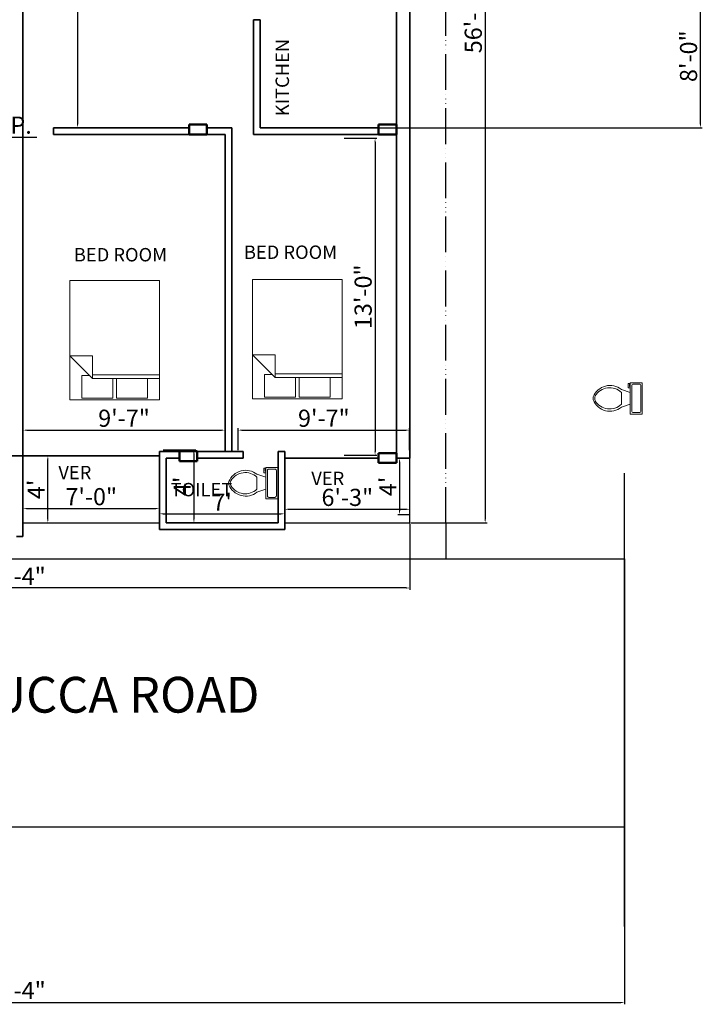
# Model space of a CAD drawing. Units: inches. Extents: x 2680 to 3617, y 1720 to 2823.
# Tile 2 of 4: x 3159 to 3617, y 1720 to 2380. Entities that reach past the tile are written whole.
import ezdxf

# ---------------------------------------------------------------- set-up
doc = ezdxf.new("R2010")
doc.units = ezdxf.units.IN
doc.linetypes.add('ACAD_ISO06W100', pattern=[36, 24, -3, 0, -3, 0, -3, 0, -3])
for name, color, linetype, lineweight in [('A-ANNO-DIMS', 2, 'Continuous', 18), ('A-ANNO-TEXT', 3, 'Continuous', 18), ('A-AREA-IDEN', 244, 'Continuous', 18), ('A-COLS', 1, 'Continuous', 50), ('A-FLOR', 7, 'Continuous', 25), ('A-FLOR-FIXT', 9, 'Continuous', 18), ('A-FURN', 8, 'Continuous', 18), ('A-WALL', 7, 'Continuous', 35), ('C-PROP', 6, 'ACAD_ISO06W100', 25), ('C-ROAD', 244, 'Continuous', 25)]:
    doc.layers.add(name, color=color, linetype=linetype, lineweight=lineweight)
doc.styles.get("Standard").update_dxf_attribs({"font": 'arial.ttf'})
doc.dimstyles.new('ISO-25', dxfattribs={"dimtxt": 11.5, "dimasz": 2.5, "dimexe": 1.25, "dimexo": 0.625, "dimtad": 1, "dimdec": 1, "dimlunit": 3, "dimtxsty": 'Standard', "dimcen": 2.5, "dimadec": 0, "dimazin": 0, "dimtfac": 1, "dimtdec": 1, "dimtmove": 0, "dimatfit": 3, "dimfxl": 1, "dimarcsym": 0})

# ---------------------------------------------------------------- blocks, each defined once
blk = doc.blocks.new('*D21')
at = {"layer": 'A-ANNO-DIMS', "color": 0, "lineweight": -2, "transparency": 16777216}
for p, q in [((3376.75, 2300.43), (3398.77, 2300.43)), ((3397.52, 2297.93), (3397.52, 2090.43)), ((3376.74, 2087.93), (3398.77, 2087.93))]:
    blk.add_line(p, q, dxfattribs=at)
at = {"layer": 'A-ANNO-DIMS', "color": 0, "lineweight": 70, "transparency": 16777216}
for points in [[(3397.11, 2297.93), (3397.94, 2297.93), (3397.52, 2300.43)], [(3397.11, 2090.43), (3397.94, 2090.43), (3397.52, 2087.93)]]:
    blk.add_solid(points, dxfattribs=at)
at = {"layer": 'Defpoints', "color": 0, "lineweight": 70, "transparency": 16777216}
for p in [(3376.13, 2300.43), (3376.11, 2087.93), (3397.52, 2087.93)]:
    blk.add_point(p, dxfattribs=at)
at = {"layer": 'A-ANNO-DIMS', "color": 0, "transparency": 16777216, "insert": (3391.02, 2194.18), "char_height": 11.5, "attachment_point": 5, "rotation": 90}
blk.add_mtext('13\'-0"', dxfattribs=at)
blk = doc.blocks.new('*D22')
at = {"layer": 'A-ANNO-DIMS', "color": 0, "lineweight": -2, "transparency": 16777216}
for p, q in [((3305.65, 2091.23), (3305.65, 2105.97)), ((3308.15, 2104.72), (3418.15, 2104.72)), ((3420.65, 2091.23), (3420.65, 2105.97))]:
    blk.add_line(p, q, dxfattribs=at)
at = {"layer": 'A-ANNO-DIMS', "color": 0, "lineweight": 70, "transparency": 16777216}
for points in [[(3308.15, 2105.14), (3308.15, 2104.31), (3305.65, 2104.72)], [(3418.15, 2105.14), (3418.15, 2104.31), (3420.65, 2104.72)]]:
    blk.add_solid(points, dxfattribs=at)
at = {"layer": 'Defpoints', "color": 0, "lineweight": 70, "transparency": 16777216}
for p in [(3420.65, 2104.72), (3305.65, 2090.6), (3420.65, 2090.6)]:
    blk.add_point(p, dxfattribs=at)
at = {"layer": 'A-ANNO-DIMS', "color": 0, "transparency": 16777216, "insert": (3363.15, 2111.22), "char_height": 11.5, "attachment_point": 5}
blk.add_mtext('9\'-7"', dxfattribs=at)
blk = doc.blocks.new('*D23')
at = {"layer": 'A-ANNO-DIMS', "color": 0, "lineweight": -2, "transparency": 16777216}
for p, q in [((3161.31, 2091.23), (3161.31, 2105.97)), ((3163.81, 2104.72), (3294.41, 2104.72)), ((3296.91, 2091.23), (3296.91, 2105.97))]:
    blk.add_line(p, q, dxfattribs=at)
at = {"layer": 'A-ANNO-DIMS', "color": 0, "lineweight": 70, "transparency": 16777216}
for points in [[(3163.81, 2105.14), (3163.81, 2104.31), (3161.31, 2104.72)], [(3294.41, 2105.14), (3294.41, 2104.31), (3296.91, 2104.72)]]:
    blk.add_solid(points, dxfattribs=at)
at = {"layer": 'Defpoints', "color": 0, "lineweight": 70, "transparency": 16777216}
for p in [(3296.91, 2104.72), (3161.31, 2090.6), (3296.91, 2090.6)]:
    blk.add_point(p, dxfattribs=at)
at = {"layer": 'A-ANNO-DIMS', "color": 0, "transparency": 16777216, "insert": (3229.11, 2111.22), "char_height": 11.5, "attachment_point": 5}
blk.add_mtext('9\'-7"', dxfattribs=at)
blk = doc.blocks.new('*D26')
at = {"layer": 'A-ANNO-DIMS', "color": 0, "lineweight": -2, "transparency": 16777216}
for p, q in [((3227.79, 2521.5), (3196.65, 2521.5)), ((3197.9, 2519), (3197.9, 2310)), ((3226.7, 2307.5), (3196.65, 2307.5))]:
    blk.add_line(p, q, dxfattribs=at)
at = {"layer": 'A-ANNO-DIMS', "color": 0, "lineweight": 70, "transparency": 16777216}
for points in [[(3197.48, 2519), (3198.31, 2519), (3197.9, 2521.5)], [(3197.48, 2310), (3198.31, 2310), (3197.9, 2307.5)]]:
    blk.add_solid(points, dxfattribs=at)
at = {"layer": 'Defpoints', "color": 0, "lineweight": 70, "transparency": 16777216}
for p in [(3228.41, 2521.5), (3197.9, 2307.5), (3227.32, 2307.5)]:
    blk.add_point(p, dxfattribs=at)
at = {"layer": 'A-ANNO-DIMS', "color": 0, "transparency": 16777216, "insert": (3191.4, 2414.5), "char_height": 11.5, "attachment_point": 5, "rotation": 90}
blk.add_mtext('17\'-10"', dxfattribs=at)
blk = doc.blocks.new('*D32')
at = {"layer": 'A-ANNO-DIMS', "color": 0, "lineweight": -2, "transparency": 16777216}
for p, q in [((3161.94, 2087.51), (3179.26, 2087.51)), ((3178.01, 2045), (3178.01, 2085.01)), ((3161.94, 2042.5), (3179.26, 2042.5))]:
    blk.add_line(p, q, dxfattribs=at)
at = {"layer": 'A-ANNO-DIMS', "color": 0, "lineweight": 70, "transparency": 16777216}
for points in [[(3177.59, 2085.01), (3178.43, 2085.01), (3178.01, 2087.51)], [(3177.59, 2045), (3178.43, 2045), (3178.01, 2042.5)]]:
    blk.add_solid(points, dxfattribs=at)
at = {"layer": 'Defpoints', "color": 0, "lineweight": 70, "transparency": 16777216}
for p in [(3161.31, 2087.51), (3178.01, 2087.51), (3161.31, 2042.5)]:
    blk.add_point(p, dxfattribs=at)
at = {"layer": 'A-ANNO-DIMS', "color": 0, "transparency": 16777216, "insert": (3171.63, 2065.01), "char_height": 11.5, "attachment_point": 5, "rotation": 90}
blk.add_mtext("4'", dxfattribs=at)
blk = doc.blocks.new('*D33')
at = {"layer": 'A-ANNO-DIMS', "color": 0, "lineweight": -2, "transparency": 16777216}
for p, q in [((3255.31, 2091.6), (3277.26, 2091.6)), ((3276.01, 2089.1), (3276.01, 2045)), ((3258.04, 2042.5), (3277.26, 2042.5))]:
    blk.add_line(p, q, dxfattribs=at)
at = {"layer": 'A-ANNO-DIMS', "color": 0, "lineweight": 70, "transparency": 16777216}
for points in [[(3275.59, 2089.1), (3276.42, 2089.1), (3276.01, 2091.6)], [(3275.59, 2045), (3276.42, 2045), (3276.01, 2042.5)]]:
    blk.add_solid(points, dxfattribs=at)
at = {"layer": 'Defpoints', "color": 0, "lineweight": 70, "transparency": 16777216}
for p in [(3254.69, 2091.6), (3257.41, 2042.5), (3276.01, 2042.5)]:
    blk.add_point(p, dxfattribs=at)
at = {"layer": 'A-ANNO-DIMS', "color": 0, "transparency": 16777216, "insert": (3269.63, 2067.05), "char_height": 11.5, "attachment_point": 5, "rotation": 90}
blk.add_mtext("4'", dxfattribs=at)
blk = doc.blocks.new('*D36')
at = {"layer": 'A-ANNO-DIMS', "color": 0, "lineweight": -2, "transparency": 16777216}
for p, q in [((3161.31, 2043.13), (3161.31, 2053.37)), ((3163.81, 2052.12), (3250.41, 2052.12)), ((3252.91, 2043.13), (3252.91, 2053.37))]:
    blk.add_line(p, q, dxfattribs=at)
at = {"layer": 'A-ANNO-DIMS', "color": 0, "lineweight": 70, "transparency": 16777216}
for points in [[(3163.81, 2052.53), (3163.81, 2051.7), (3161.31, 2052.12)], [(3250.41, 2052.53), (3250.41, 2051.7), (3252.91, 2052.12)]]:
    blk.add_solid(points, dxfattribs=at)
at = {"layer": 'Defpoints', "color": 0, "lineweight": 70, "transparency": 16777216}
for p in [(3252.91, 2052.12), (3161.31, 2042.5), (3252.91, 2042.5)]:
    blk.add_point(p, dxfattribs=at)
at = {"layer": 'A-ANNO-DIMS', "color": 0, "transparency": 16777216, "insert": (3207.11, 2058.61), "char_height": 11.5, "attachment_point": 5}
blk.add_mtext('7\'-0"', dxfattribs=at)
blk = doc.blocks.new('*D37')
at = {"layer": 'A-ANNO-DIMS', "color": 0, "lineweight": -2, "transparency": 16777216}
for p, q in [((3252.91, 2043.13), (3252.91, 2049.87)), ((3255.41, 2048.62), (3334.41, 2048.62)), ((3336.91, 2043.13), (3336.91, 2049.87))]:
    blk.add_line(p, q, dxfattribs=at)
at = {"layer": 'A-ANNO-DIMS', "color": 0, "lineweight": 70, "transparency": 16777216}
for points in [[(3255.41, 2049.03), (3255.41, 2048.2), (3252.91, 2048.62)], [(3334.41, 2049.03), (3334.41, 2048.2), (3336.91, 2048.62)]]:
    blk.add_solid(points, dxfattribs=at)
at = {"layer": 'Defpoints', "color": 0, "lineweight": 70, "transparency": 16777216}
for p in [(3336.91, 2048.62), (3252.91, 2042.5), (3336.91, 2042.5)]:
    blk.add_point(p, dxfattribs=at)
at = {"layer": 'A-ANNO-DIMS', "color": 0, "transparency": 16777216, "insert": (3294.91, 2054.99), "char_height": 11.5, "attachment_point": 5}
blk.add_mtext("7'", dxfattribs=at)
blk = doc.blocks.new('*D38')
at = {"layer": 'A-ANNO-DIMS', "color": 0, "lineweight": -2, "transparency": 16777216}
for p, q in [((3336.91, 2043.13), (3336.91, 2052.9)), ((3339.41, 2051.65), (3418.41, 2051.65)), ((3420.91, 2043.13), (3420.91, 2052.9))]:
    blk.add_line(p, q, dxfattribs=at)
at = {"layer": 'A-ANNO-DIMS', "color": 0, "lineweight": 70, "transparency": 16777216}
for points in [[(3339.41, 2052.07), (3339.41, 2051.23), (3336.91, 2051.65)], [(3418.41, 2052.07), (3418.41, 2051.23), (3420.91, 2051.65)]]:
    blk.add_solid(points, dxfattribs=at)
at = {"layer": 'Defpoints', "color": 0, "lineweight": 70, "transparency": 16777216}
for p in [(3420.91, 2051.65), (3336.91, 2042.5), (3420.91, 2042.5)]:
    blk.add_point(p, dxfattribs=at)
at = {"layer": 'A-ANNO-DIMS', "color": 0, "transparency": 16777216, "insert": (3378.91, 2058.15), "char_height": 11.5, "attachment_point": 5}
blk.add_mtext('6\'-3"', dxfattribs=at)
blk = doc.blocks.new('*D39')
at = {"layer": 'A-ANNO-DIMS', "color": 0, "lineweight": -2, "transparency": 16777216}
for p, q in [((3420.29, 2086), (3412.7, 2086)), ((3413.95, 2083.5), (3413.95, 2050.52)), ((3420.29, 2048.02), (3412.7, 2048.02))]:
    blk.add_line(p, q, dxfattribs=at)
at = {"layer": 'A-ANNO-DIMS', "color": 0, "lineweight": 70, "transparency": 16777216}
for points in [[(3413.53, 2083.5), (3414.36, 2083.5), (3413.95, 2086)], [(3413.53, 2050.52), (3414.36, 2050.52), (3413.95, 2048.02)]]:
    blk.add_solid(points, dxfattribs=at)
at = {"layer": 'Defpoints', "color": 0, "lineweight": 70, "transparency": 16777216}
for p in [(3420.91, 2086), (3413.95, 2048.02), (3420.91, 2048.02)]:
    blk.add_point(p, dxfattribs=at)
at = {"layer": 'A-ANNO-DIMS', "color": 0, "transparency": 16777216, "insert": (3407.57, 2067.01), "char_height": 11.5, "attachment_point": 5, "rotation": 90}
blk.add_mtext("4'", dxfattribs=at)
blk = doc.blocks.new('*D40')
at = {"layer": 'A-ANNO-DIMS', "color": 0, "lineweight": -2, "transparency": 16777216}
for p, q in [((2888.91, 2041.88), (2888.91, 1997.63)), ((3420.91, 2041.88), (3420.91, 1997.63)), ((3418.41, 1998.88), (2891.41, 1998.88))]:
    blk.add_line(p, q, dxfattribs=at)
at = {"layer": 'A-ANNO-DIMS', "color": 0, "lineweight": 70, "transparency": 16777216}
for points in [[(2891.41, 1999.29), (2891.41, 1998.46), (2888.91, 1998.88)], [(3418.41, 1999.29), (3418.41, 1998.46), (3420.91, 1998.88)]]:
    blk.add_solid(points, dxfattribs=at)
at = {"layer": 'Defpoints', "color": 0, "lineweight": 70, "transparency": 16777216}
for p in [(2888.91, 2042.5), (3420.91, 2042.5), (2888.91, 1998.88)]:
    blk.add_point(p, dxfattribs=at)
at = {"layer": 'A-ANNO-DIMS', "color": 0, "transparency": 16777216, "insert": (3154.91, 2005.25), "char_height": 11.5, "attachment_point": 5}
blk.add_mtext('44\'-4"', dxfattribs=at)
blk = doc.blocks.new('*D43')
at = {"layer": 'A-ANNO-DIMS', "color": 0, "lineweight": -2, "transparency": 16777216}
for p, q in [((3421.54, 2724.5), (3472.64, 2724.5)), ((3471.39, 2722), (3471.39, 2045)), ((3421.54, 2042.5), (3472.64, 2042.5))]:
    blk.add_line(p, q, dxfattribs=at)
at = {"layer": 'A-ANNO-DIMS', "color": 0, "lineweight": 70, "transparency": 16777216}
for points in [[(3470.98, 2722), (3471.81, 2722), (3471.39, 2724.5)], [(3470.98, 2045), (3471.81, 2045), (3471.39, 2042.5)]]:
    blk.add_solid(points, dxfattribs=at)
at = {"layer": 'Defpoints', "color": 0, "lineweight": 70, "transparency": 16777216}
for p in [(3420.91, 2724.5), (3420.91, 2042.5), (3471.39, 2042.5)]:
    blk.add_point(p, dxfattribs=at)
at = {"layer": 'A-ANNO-DIMS', "color": 0, "transparency": 16777216, "insert": (3464.9, 2383.5), "char_height": 11.5, "attachment_point": 5, "rotation": 90}
blk.add_mtext('56\'-10"', dxfattribs=at)
blk = doc.blocks.new('Bed - Queen')
for p, q in [((0, -80.00003), (0, 0)), ((0, 0), (59.99999, 0)), ((59.99999, 0), (59.99999, -80.00003)), ((7.99999, -1.2), (28.79998, -1.2)), ((7.99999, -14.4), (7.99999, -1.2)), ((28.79998, -1.2), (28.79998, -14.4)), ((31.19999, -1.2), (51.99999, -1.2)), ((31.19999, -14.4), (31.19999, -1.2)), ((51.99999, -1.2), (51.99999, -16.4)), ((0, -14.4), (44.8, -14.4)), ((44.8, -16.8), (0, -16.8)), ((59.99999, -29.6), (44.8, -14.4)), ((44.8, -14.4), (44.8, -29.6)), ((51.99999, -16.4), (46.79936, -16.4)), ((44.8, -29.6), (59.99999, -29.6)), ((59.99999, -80.00003), (0, -80.00003))]:
    blk.add_line(p, q)
blk = doc.blocks.new('Toilet - top')
for p, q in [((9.5, -6), (9.5, -2)), ((-10, -8.5), (-8, -8.5)), ((-10, -9.5), (-10, -8.5)), ((-7, -9.5), (-10, -9.5)), ((-8, -8.5), (-8, -8)), ((-7, -8), (-7, -9.5)), ((-4, -8), (-6, -14)), ((4, -8), (6, -14)), ((4, -14), (-4, -14))]:
    blk.add_line(p, q)
blk.add_lwpolyline([(10.5, -8), (10.5, 0), (-10.5, 0), (-10.5, -8)], close=True)
for points in [[(-9.5, -2), (-9.5, -6)], [(8.5, -1), (-8.5, -1)], [(-8.5, -7), (8.5, -7)]]:
    blk.add_lwpolyline(points)
for centre, radius, start, end in [((-8.62, -1.88), 0.884, 81.8699, 188.1301), ((-8.62, -6.12), 0.884, 171.8699, 278.1301), ((8.62, -1.88), 0.884, 351.8699, 98.1301), ((8.62, -6.12), 0.884, 261.8699, 8.1301), ((3.52, -21.58), 12.17, 141.46911, 247.97143), ((4.2, -21.82), 11.33, 136.36773, 238.94682), ((-3.52, -21.58), 12.17, 292.02843, 38.53071), ((-4.2, -21.82), 11.33, 301.05301, 43.63209), ((0, -27.88), 4, 245.73182, 294.26817), ((0, -29), 4, 254.86053, 285.13947)]:
    blk.add_arc(centre, radius, start, end)
blk = doc.blocks.new('COL-12X6P64')
for p, q in [((0, 0), (0, 6.64)), ((0, 6.64), (12, 6.64)), ((12, 6.64), (12, 0)), ((12, 0), (0, 0))]:
    blk.add_line(p, q)
blk = doc.blocks.new('*D58')
at = {"layer": 'A-ANNO-DIMS', "color": 0, "lineweight": -2, "transparency": 16777216}
for p, q in [((3032.31, 2302.38), (3032.31, 2299.95)), ((3034.81, 2301.2), (3041.81, 2301.2)), ((3044.31, 2302.38), (3044.31, 2299.95)), ((3044.31, 2301.2), (3170.7, 2301.2))]:
    blk.add_line(p, q, dxfattribs=at)
at = {"layer": 'A-ANNO-DIMS', "color": 0, "lineweight": 70, "transparency": 16777216}
for points in [[(3034.81, 2301.62), (3034.81, 2300.79), (3032.31, 2301.2)], [(3041.81, 2301.62), (3041.81, 2300.79), (3044.31, 2301.2)]]:
    blk.add_solid(points, dxfattribs=at)
at = {"layer": 'Defpoints', "color": 0, "lineweight": 70, "transparency": 16777216}
for p in [(3032.31, 2303), (3044.31, 2303), (3044.31, 2301.2)]:
    blk.add_point(p, dxfattribs=at)
at = {"layer": 'A-ANNO-DIMS', "color": 0, "transparency": 16777216, "insert": (3108.75, 2307.78), "char_height": 11.5, "attachment_point": 5}
blk.add_mtext('COL A 1\'-0" TYP.', dxfattribs=at)
blk = doc.blocks.new('*D70')
at = {"layer": 'A-ANNO-DIMS', "color": 0, "lineweight": -2, "transparency": 16777216}
for p, q in [((2744.91, 1837.88), (2744.91, 1719.69)), ((3564.91, 1837.88), (3564.91, 1719.69)), ((2747.41, 1720.94), (3562.41, 1720.94))]:
    blk.add_line(p, q, dxfattribs=at)
at = {"layer": 'A-ANNO-DIMS', "color": 0, "lineweight": 70, "transparency": 16777216}
for points in [[(2747.41, 1721.36), (2747.41, 1720.52), (2744.91, 1720.94)], [(3562.41, 1721.36), (3562.41, 1720.52), (3564.91, 1720.94)]]:
    blk.add_solid(points, dxfattribs=at)
at = {"layer": 'Defpoints', "color": 0, "lineweight": 70, "transparency": 16777216}
for p in [(2744.91, 1838.5), (3564.91, 1838.5), (3564.91, 1720.94)]:
    blk.add_point(p, dxfattribs=at)
at = {"layer": 'A-ANNO-DIMS', "color": 0, "transparency": 16777216, "insert": (3154.91, 1727.44), "char_height": 11.5, "attachment_point": 5}
blk.add_mtext('68\'-4"', dxfattribs=at)
blk = doc.blocks.new('*D74')
at = {"layer": 'A-ANNO-DIMS', "color": 0, "lineweight": -2, "transparency": 16777216}
for p, q in [((3412.54, 2403.5), (3617.06, 2403.5)), ((3615.81, 2310), (3615.81, 2401)), ((3321.04, 2307.5), (3617.06, 2307.5))]:
    blk.add_line(p, q, dxfattribs=at)
at = {"layer": 'A-ANNO-DIMS', "color": 0, "lineweight": 70, "transparency": 16777216}
for points in [[(3615.4, 2401), (3616.23, 2401), (3615.81, 2403.5)], [(3615.4, 2310), (3616.23, 2310), (3615.81, 2307.5)]]:
    blk.add_solid(points, dxfattribs=at)
at = {"layer": 'Defpoints', "color": 0, "lineweight": 70, "transparency": 16777216}
for p in [(3411.91, 2403.5), (3615.81, 2403.5), (3320.41, 2307.5)]:
    blk.add_point(p, dxfattribs=at)
at = {"layer": 'A-ANNO-DIMS', "color": 0, "transparency": 16777216, "insert": (3609.32, 2355.5), "char_height": 11.5, "attachment_point": 5, "rotation": 90}
blk.add_mtext('8\'-0"', dxfattribs=at)

msp = doc.modelspace()

# ---------------------------------------------------------------- linework, layer by layer
at = {"layer": 'A-FLOR'}
for p, q in [((3420.91, 2042.5), (3420.91, 2086)), ((3161.31, 2042.5), (3252.91, 2042.5)), ((3336.91, 2042.5), (3420.91, 2042.5))]:
    msp.add_line(p, q, dxfattribs=at)
at = {"layer": 'A-WALL'}
for p, q in [((3420.91, 2724.5), (3420.91, 2086)), ((3411.91, 2715.5), (3411.91, 2086)), ((3161.31, 2521.5), (3161.31, 2042.5)), ((3315.91, 2379.98), (3320.41, 2379.98)), ((3315.91, 2379.98), (3315.91, 2303)), ((3320.41, 2379.98), (3320.41, 2307.5)), ((3181.91, 2307.5), (3181.91, 2303)), ((3181.91, 2307.5), (3272.73, 2307.5)), ((3284.73, 2307.5), (3301.41, 2307.5)), ((3301.41, 2307.5), (3301.41, 2090.5)), ((3320.41, 2307.5), (3399.87, 2307.5)), ((3320.41, 2307.5), (3399.87, 2307.5)), ((3411.87, 2307.5), (3411.91, 2307.5)), ((3411.87, 2307.5), (3411.91, 2307.5)), ((3181.91, 2303), (3296.91, 2303)), ((3296.91, 2303), (3296.91, 2090.5)), ((3315.91, 2303), (3411.91, 2303)), ((3315.91, 2303), (3411.91, 2303)), ((3056.91, 2087.51), (3252.91, 2087.51)), ((3252.91, 2090.5), (3252.91, 2038)), ((3309.06, 2090.5), (3252.91, 2090.5)), ((3309.06, 2090.5), (3309.06, 2086)), ((3332.41, 2090.5), (3332.41, 2042.5)), ((3336.91, 2090.5), (3332.41, 2090.5)), ((3336.91, 2090.5), (3336.91, 2038)), ((3257.41, 2086), (3257.41, 2042.5)), ((3266.28, 2086), (3257.41, 2086)), ((3309.06, 2086), (3278.28, 2086)), ((3399.86, 2086), (3336.91, 2086)), ((3420.91, 2086), (3411.86, 2086)), ((3161.31, 2033.5), (3161.31, 2042.5)), ((3332.41, 2042.5), (3257.41, 2042.5)), ((3336.91, 2038), (3252.91, 2038)), ((3156.91, 2033.5), (3161.31, 2033.5))]:
    msp.add_line(p, q, dxfattribs=at)
at = {"layer": 'C-PROP'}
for q in [(3444.91, 2724.5), (3444.91, 2018.5)]:
    msp.add_line((3444.91, 2042.5), q, dxfattribs=at)
at = {"layer": 'C-ROAD'}
msp.add_line((3564.91, 1838.5), (3564.91, 1771.84), dxfattribs=at)
for points in [[(2744.91, 1771.84), (2744.91, 1838.5), (2744.91, 2018.5), (2804.91, 2018.5), (2984.91, 2018.5), (3444.91, 2018.5), (3504.91, 2018.5), (3564.91, 2018.5), (3564.91, 2075.96)], [(3564.91, 1771.84), (3564.91, 2018.5), (3564.91, 1838.5), (3504.91, 1838.5), (3444.91, 1838.5), (2984.91, 1838.5), (2804.91, 1838.5), (2744.91, 1838.5)]]:
    msp.add_lwpolyline(points, dxfattribs=at)

# ---------------------------------------------------------------- block references
at = {"layer": 'A-COLS'}
for p in [(3272.73, 2303), (3399.87, 2303), (3266.28, 2083.89), (3399.86, 2082.75)]:
    msp.add_blockref('COL-12X6P64', p, dxfattribs=at)
at = {"layer": 'A-FLOR-FIXT', "rotation": 270}
for p in [(3576.77, 2126.04), (3332.3, 2069.16)]:
    msp.add_blockref('Toilet - top', p, dxfattribs=at)
at = {"layer": 'A-FURN', "rotation": 180}
for p in [(3375.37, 2125.67), (3252.83, 2125)]:
    msp.add_blockref('Bed - Queen', p, dxfattribs=at)

# ---------------------------------------------------------------- texts
at = {"layer": 'A-ANNO-TEXT', "insert": (2933.78, 1954.28), "char_height": 9, "attachment_point": 1}
msp.add_mtext_dynamic_manual_height_columns('\'\\P{\\H2.66667x;15\'-0" WIDE PUCCA ROAD}', width=461.2944, gutter_width=12.5, heights=[0], dxfattribs=at)
at = {"layer": 'A-AREA-IDEN', "insert": (3330.79, 2315.3), "char_height": 9, "attachment_point": 1, "rotation": 90}
msp.add_mtext_dynamic_manual_height_columns('{KITCHEN}', width=87.2951, gutter_width=12.5, heights=[0], dxfattribs=at)
at = {"layer": 'A-AREA-IDEN', "char_height": 9, "attachment_point": 1}
for s, insert in [('{BED ROOM}', (3195.47, 2226.88)), ('{BED ROOM}', (3309.56, 2228.55)), ('{VER}', (3185.08, 2080.78)), ('{VER}', (3354.75, 2076.85)), ('{TOILET}', (3260.43, 2069.35))]:
    msp.add_mtext_dynamic_manual_height_columns(s, width=87.2951, gutter_width=12.5, heights=[0], dxfattribs=dict(at, insert=insert))

# ---------------------------------------------------------------- dimensions: what is measured, and where the dimension line sits
at = {"layer": 'A-ANNO-DIMS'}
for base, p1, p2, override, picture, middle in [((3471.39, 2042.5), (3420.91, 2724.5), (3420.91, 2042.5), {"dimclrd": 0, "dimclre": 0, "dimclrt": 0}, '*D43', (3464.9, 2383.5)), ((3197.9, 2307.5), (3228.41, 2521.5), (3227.32, 2307.5), {"dimclrd": 0, "dimclre": 0, "dimclrt": 0}, '*D26', (3191.4, 2414.5)), ((3615.81, 2403.5), (3320.41, 2307.5), (3411.91, 2403.5), {"dimdec": 1, "dimlfac": 1, "dimrnd": 0, "dimzin": 1, "dimdsep": 46, "dimlunit": 4, "dimfrac": 2}, '*D74', (3609.32, 2355.5))]:
    dim = msp.add_linear_dim(base=base, p1=p1, p2=p2, angle=90, dimstyle='ISO-25', override=override, dxfattribs=at)
    dim.commit()
    dim.dimension.update_dxf_attribs({"geometry": picture, "text_midpoint": middle})
for base, p1, p2, text, override, picture, middle in [((3044.31, 2301.2), (3032.31, 2303), (3044.31, 2303), 'COL A <> TYP.', {"dimdec": 1, "dimlfac": 1, "dimrnd": 0, "dimzin": 1, "dimdsep": 46, "dimlunit": 4, "dimfrac": 2}, '*D58', (3108.75, 2307.78)), ((3296.91, 2104.72), (3161.31, 2090.6), (3296.91, 2090.6), '9\'-7"', {"dimclrd": 0, "dimclre": 0, "dimclrt": 0}, '*D23', (3229.11, 2111.22)), ((3252.91, 2052.12), (3161.31, 2042.5), (3252.91, 2042.5), '7\'-0"', {"dimclrd": 0, "dimclre": 0, "dimclrt": 0}, '*D36', (3207.11, 2058.61)), ((3420.91, 2051.65), (3336.91, 2042.5), (3420.91, 2042.5), '6\'-3"', {"dimclrd": 0, "dimclre": 0, "dimclrt": 0}, '*D38', (3378.91, 2058.15))]:
    dim = msp.add_linear_dim(base=base, p1=p1, p2=p2, text=text, dimstyle='ISO-25', override=override, dxfattribs=at)
    dim.commit()
    dim.dimension.update_dxf_attribs({"geometry": picture, "text_midpoint": middle})
for base, p1, p2, text, picture, middle in [((3397.52, 2087.93), (3376.13, 2300.43), (3376.11, 2087.93), '13\'-0"', '*D21', (3391.02, 2194.18)), ((3178.01, 2087.51), (3161.31, 2042.5), (3161.31, 2087.51), "4'", '*D32', (3171.63, 2065.01)), ((3276.01, 2042.5), (3254.69, 2091.6), (3257.41, 2042.5), "4'", '*D33', (3269.63, 2067.05)), ((3413.95, 2048.02), (3420.91, 2086), (3420.91, 2048.02), "4'", '*D39', (3407.57, 2067.01))]:
    dim = msp.add_linear_dim(base=base, p1=p1, p2=p2, angle=90, text=text, dimstyle='ISO-25', override={"dimclrd": 0, "dimclre": 0, "dimclrt": 0}, dxfattribs=at)
    dim.commit()
    dim.dimension.update_dxf_attribs({"geometry": picture, "text_midpoint": middle})
for base, p1, p2, override, picture, middle in [((3420.65, 2104.72), (3305.65, 2090.6), (3420.65, 2090.6), {"dimclrd": 0, "dimclre": 0, "dimclrt": 0}, '*D22', (3363.15, 2111.22)), ((3336.91, 2048.62), (3252.91, 2042.5), (3336.91, 2042.5), {"dimclrd": 0, "dimclre": 0, "dimclrt": 0}, '*D37', (3294.91, 2054.99)), ((2888.91, 1998.88), (3420.91, 2042.5), (2888.91, 2042.5), {"dimclrd": 0, "dimclre": 0, "dimclrt": 0}, '*D40', (3154.91, 2005.25)), ((3564.91, 1720.94), (2744.91, 1838.5), (3564.91, 1838.5), {"dimdec": 1, "dimlfac": 1, "dimrnd": 0, "dimzin": 1, "dimdsep": 46, "dimlunit": 4, "dimfrac": 2}, '*D70', (3154.91, 1727.44))]:
    dim = msp.add_linear_dim(base=base, p1=p1, p2=p2, dimstyle='ISO-25', override=override, dxfattribs=at)
    dim.commit()
    dim.dimension.update_dxf_attribs({"geometry": picture, "text_midpoint": middle})

doc.saveas('drawing.dxf')
